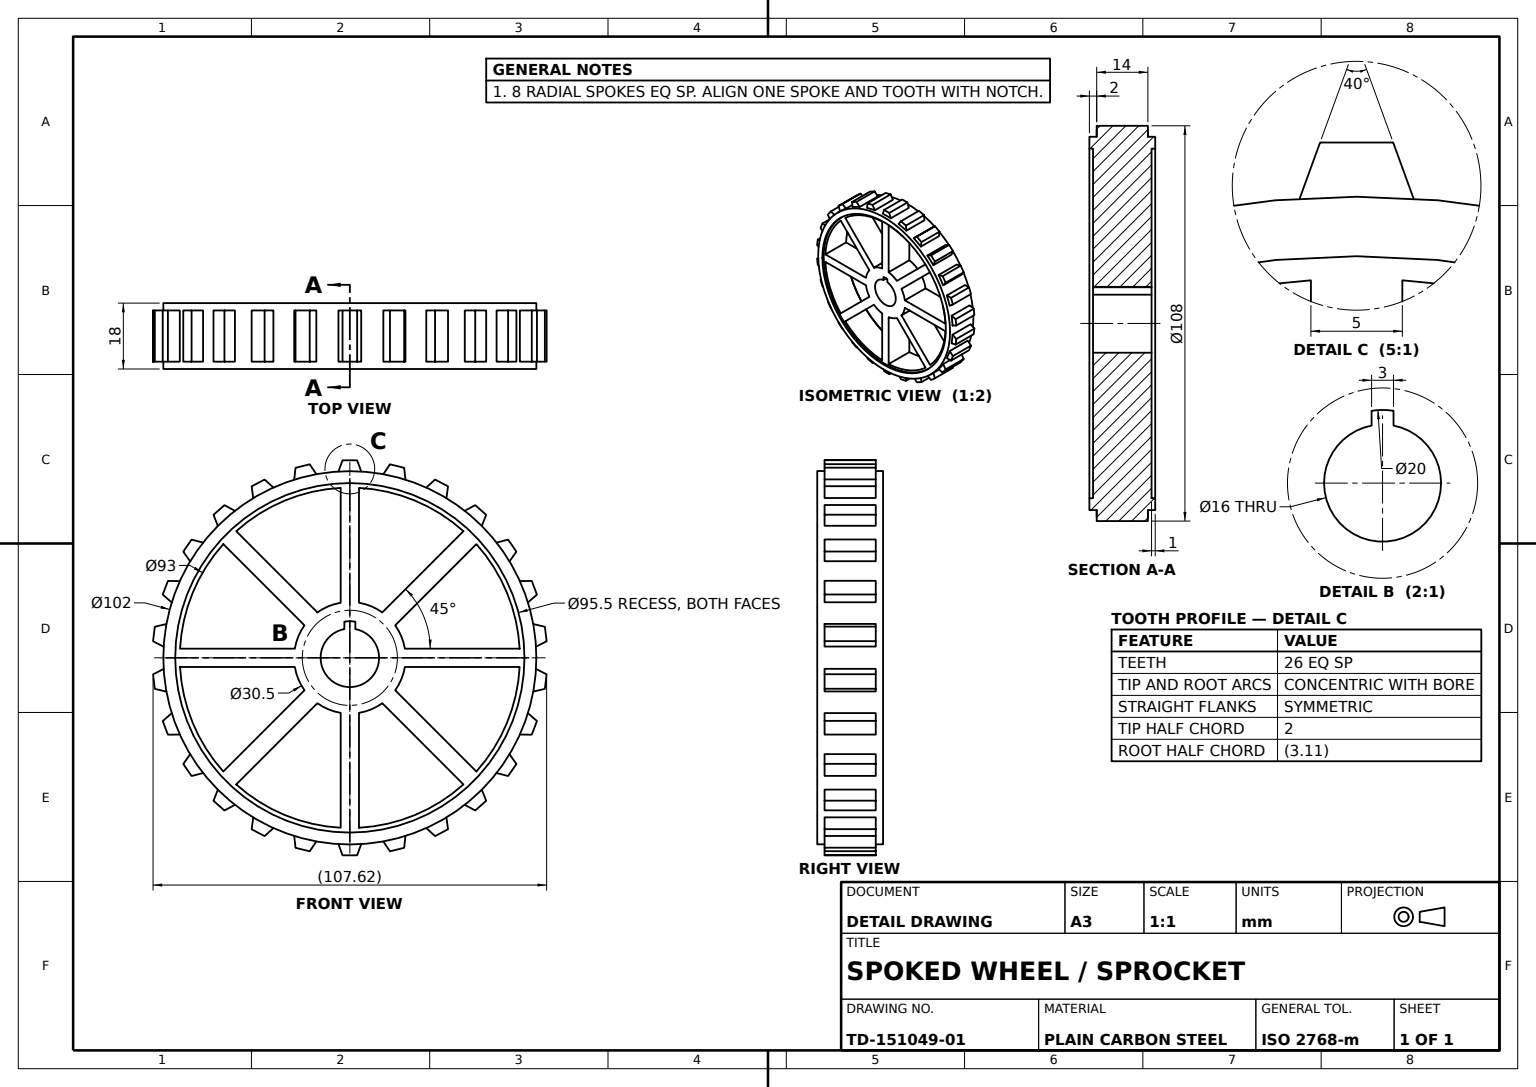
SolidWorks part; units mm, degrees
material "Plain Carbon Steel"
ref_plane "Front Plane" through (0, 0, 0) normal (0, 0, 1) x (1, 0, 0)
ref_plane "Top Plane" through (0, 0, 0) normal (0, 1, 0) x (1, 0, 0)
ref_plane "Right Plane" through (0, 0, 0) normal (1, 0, 0) x (0, 0, -1)
sketch "Hub Spokes Rim Sketch" plane through (0, 0, 0) normal (0, 0, 1) x (1, 0, 0)
  line L0 (0, 0) -> (0, 62.7961) construction
  line L1 (-2.5, 15.0437) -> (-2.5, 46.4327)
  line L2 (2.5, 46.4327) -> (2.5, 15.0437)
  line L3 (34.6007, 31.0651) -> (12.4053, 8.8697)
  line L4 (8.8697, 12.4053) -> (31.0651, 34.6007)
  line L5 (46.4327, -2.5) -> (15.0437, -2.5)
  line L6 (15.0437, 2.5) -> (46.4327, 2.5)
  line L7 (31.0651, -34.6007) -> (8.8697, -12.4053)
  line L8 (12.4053, -8.8697) -> (34.6007, -31.0651)
  line L9 (-2.5, -46.4327) -> (-2.5, -15.0437)
  line L10 (2.5, -15.0437) -> (2.5, -46.4327)
  line L11 (-34.6007, -31.0651) -> (-12.4053, -8.8697)
  line L12 (-8.8697, -12.4053) -> (-31.0651, -34.6007)
  line L13 (-46.4327, 2.5) -> (-15.0437, 2.5)
  line L14 (-15.0437, -2.5) -> (-46.4327, -2.5)
  line L15 (-31.0651, 34.6007) -> (-8.8697, 12.4053)
  line L16 (-12.4053, 8.8697) -> (-34.6007, 31.0651)
  circle A0 centre (0, 0) radius 51
  arc A1 (-2.5, 15.0437) -> (-8.8697, 12.4053) centre (0, 0) ccw
  circle A2 centre (0, 0) radius 8
  arc A3 (-2.5, 46.4327) -> (-31.0651, 34.6007) centre (0, 0) ccw
  arc A4 (8.8697, 12.4053) -> (2.5, 15.0437) centre (0, 0) ccw
  arc A5 (15.0437, 2.5) -> (12.4053, 8.8697) centre (0, 0) ccw
  arc A6 (12.4053, -8.8697) -> (15.0437, -2.5) centre (0, 0) ccw
  arc A7 (2.5, -15.0437) -> (8.8697, -12.4053) centre (0, 0) ccw
  arc A8 (-8.8697, -12.4053) -> (-2.5, -15.0437) centre (0, 0) ccw
  arc A9 (-15.0437, -2.5) -> (-12.4053, -8.8697) centre (0, 0) ccw
  arc A10 (-12.4053, 8.8697) -> (-15.0437, 2.5) centre (0, 0) ccw
  arc A11 (31.0651, 34.6007) -> (2.5, 46.4327) centre (0, 0) ccw
  arc A12 (46.4327, 2.5) -> (34.6007, 31.0651) centre (0, 0) ccw
  arc A13 (34.6007, -31.0651) -> (46.4327, -2.5) centre (0, 0) ccw
  arc A14 (2.5, -46.4327) -> (31.0651, -34.6007) centre (0, 0) ccw
  arc A15 (-31.0651, -34.6007) -> (-2.5, -46.4327) centre (0, 0) ccw
  arc A16 (-46.4327, -2.5) -> (-34.6007, -31.0651) centre (0, 0) ccw
  arc A17 (-34.6007, 31.0651) -> (-46.4327, 2.5) centre (0, 0) ccw
  point P41 (0, 0)
  dimension "D1" = 16
  dimension "D2" = 30.5
  dimension "D3" = 93
  dimension "D4" = 102
  dimension "D5" = 5
  dimension "D6" = 2.5
  dimension "D7" = 8
extrude "Wheel Body 8 Spokes" add sketch "Hub Spokes Rim Sketch" along normal mid plane 18 contours L14 A16 L11 A9
sketch "Teeth Profile Sketch 26x" plane through (0, 0, 0) normal (0, 0, 1) x (1, 0, 0)
  line L0 (10.9723, 52.8735) -> (9.1598, 50.1707)
  line L1 (-2, 53.963) -> (-3.113, 50.9049)
  line L2 (2, 53.963) -> (3.113, 50.9049)
  line L3 (14.8561, 51.9163) -> (15.2049, 48.6807)
  line L4 (23.3069, 48.7113) -> (20.9002, 46.5208)
  line L5 (26.8487, 46.8524) -> (26.4131, 43.6274)
  line L6 (34.287, 41.7181) -> (31.4261, 40.1672)
  line L7 (37.2811, 39.0656) -> (36.0863, 36.0385)
  line L8 (43.2745, 32.3004) -> (40.1255, 31.4793)
  line L9 (45.5468, 29.0085) -> (43.6623, 26.3553)
  line L10 (49.747, 21.0056) -> (46.493, 20.9619)
  line L11 (51.1654, 17.2655) -> (48.7008, 15.1404)
  line L12 (53.3284, 8.4899) -> (50.1585, 9.2262)
  line L13 (53.8106, 4.5191) -> (50.909, 3.0456)
  line L14 (53.8106, -4.5191) -> (50.909, -3.0456)
  line L15 (53.3284, -8.4899) -> (50.1585, -9.2262)
  line L16 (51.1654, -17.2655) -> (48.7008, -15.1404)
  line L17 (49.747, -21.0056) -> (46.493, -20.9619)
  line L18 (45.5468, -29.0085) -> (43.6623, -26.3553)
  line L19 (43.2745, -32.3004) -> (40.1255, -31.4793)
  line L20 (37.2811, -39.0656) -> (36.0863, -36.0385)
  line L21 (34.287, -41.7181) -> (31.4261, -40.1672)
  line L22 (26.8487, -46.8524) -> (26.4131, -43.6274)
  line L23 (23.3069, -48.7113) -> (20.9002, -46.5208)
  line L24 (14.8561, -51.9163) -> (15.2049, -48.6807)
  line L25 (10.9723, -52.8735) -> (9.1598, -50.1707)
  line L26 (2, -53.963) -> (3.113, -50.9049)
  line L27 (-2, -53.963) -> (-3.113, -50.9049)
  line L28 (-10.9723, -52.8735) -> (-9.1598, -50.1707)
  line L29 (-14.8561, -51.9163) -> (-15.2049, -48.6807)
  line L30 (-23.3069, -48.7113) -> (-20.9002, -46.5208)
  line L31 (-26.8487, -46.8524) -> (-26.4131, -43.6274)
  line L32 (-34.287, -41.7181) -> (-31.4261, -40.1672)
  line L33 (-37.2811, -39.0656) -> (-36.0863, -36.0385)
  line L34 (-43.2745, -32.3004) -> (-40.1255, -31.4793)
  line L35 (-45.5468, -29.0085) -> (-43.6623, -26.3553)
  line L36 (-49.747, -21.0056) -> (-46.493, -20.9619)
  line L37 (-51.1654, -17.2655) -> (-48.7008, -15.1404)
  line L38 (-53.3284, -8.4899) -> (-50.1585, -9.2262)
  line L39 (-53.8106, -4.5191) -> (-50.909, -3.0456)
  line L40 (-53.8106, 4.5191) -> (-50.909, 3.0456)
  line L41 (-53.3284, 8.4899) -> (-50.1585, 9.2262)
  line L42 (-51.1654, 17.2655) -> (-48.7008, 15.1404)
  line L43 (-49.747, 21.0056) -> (-46.493, 20.9619)
  line L44 (-45.5468, 29.0085) -> (-43.6623, 26.3553)
  line L45 (-43.2745, 32.3004) -> (-40.1255, 31.4793)
  line L46 (-37.2811, 39.0656) -> (-36.0863, 36.0385)
  line L47 (-34.287, 41.7181) -> (-31.4261, 40.1672)
  line L48 (-26.8487, 46.8524) -> (-26.4131, 43.6274)
  line L49 (-23.3069, 48.7113) -> (-20.9002, 46.5208)
  line L50 (-14.8561, 51.9163) -> (-15.2049, 48.6807)
  line L51 (-10.9723, 52.8735) -> (-9.1598, 50.1707)
  arc A0 (2, 53.963) -> (-2, 53.963) centre (0, 0) ccw
  circle A1 centre (0, 0) radius 51 construction
  arc A2 (-3.113, 50.9049) -> (-9.1598, 50.1707) centre (0, 0) ccw
  arc A3 (14.8561, 51.9163) -> (10.9723, 52.8735) centre (0, 0) ccw
  arc A4 (26.8487, 46.8524) -> (23.3069, 48.7113) centre (0, 0) ccw
  arc A5 (37.2811, 39.0656) -> (34.287, 41.7181) centre (0, 0) ccw
  arc A6 (45.5468, 29.0085) -> (43.2745, 32.3004) centre (0, 0) ccw
  arc A7 (51.1654, 17.2655) -> (49.747, 21.0056) centre (0, 0) ccw
  arc A8 (53.8106, 4.5191) -> (53.3284, 8.4899) centre (0, 0) ccw
  arc A9 (53.3284, -8.4899) -> (53.8106, -4.5191) centre (0, 0) ccw
  arc A10 (49.747, -21.0056) -> (51.1654, -17.2655) centre (0, 0) ccw
  arc A11 (43.2745, -32.3004) -> (45.5468, -29.0085) centre (0, 0) ccw
  arc A12 (34.287, -41.7181) -> (37.2811, -39.0656) centre (0, 0) ccw
  arc A13 (23.3069, -48.7113) -> (26.8487, -46.8524) centre (0, 0) ccw
  arc A14 (10.9723, -52.8735) -> (14.8561, -51.9163) centre (0, 0) ccw
  arc A15 (-2, -53.963) -> (2, -53.963) centre (0, 0) ccw
  arc A16 (-14.8561, -51.9163) -> (-10.9723, -52.8735) centre (0, 0) ccw
  arc A17 (-26.8487, -46.8524) -> (-23.3069, -48.7113) centre (0, 0) ccw
  arc A18 (-37.2811, -39.0656) -> (-34.287, -41.7181) centre (0, 0) ccw
  arc A19 (-45.5468, -29.0085) -> (-43.2745, -32.3004) centre (0, 0) ccw
  arc A20 (-51.1654, -17.2655) -> (-49.747, -21.0056) centre (0, 0) ccw
  arc A21 (-53.8106, -4.5191) -> (-53.3284, -8.4899) centre (0, 0) ccw
  arc A22 (-53.3284, 8.4899) -> (-53.8106, 4.5191) centre (0, 0) ccw
  arc A23 (-49.747, 21.0056) -> (-51.1654, 17.2655) centre (0, 0) ccw
  arc A24 (-43.2745, 32.3004) -> (-45.5468, 29.0085) centre (0, 0) ccw
  arc A25 (-34.287, 41.7181) -> (-37.2811, 39.0656) centre (0, 0) ccw
  arc A26 (-23.3069, 48.7113) -> (-26.8487, 46.8524) centre (0, 0) ccw
  arc A27 (-10.9723, 52.8735) -> (-14.8561, 51.9163) centre (0, 0) ccw
  arc A28 (-15.2049, 48.6807) -> (-20.9002, 46.5208) centre (0, 0) ccw
  arc A29 (-26.4131, 43.6274) -> (-31.4261, 40.1672) centre (0, 0) ccw
  arc A30 (-36.0863, 36.0385) -> (-40.1255, 31.4793) centre (0, 0) ccw
  arc A31 (-43.6623, 26.3553) -> (-46.493, 20.9619) centre (0, 0) ccw
  arc A32 (-48.7008, 15.1404) -> (-50.1585, 9.2262) centre (0, 0) ccw
  arc A33 (-50.909, 3.0456) -> (-50.909, -3.0456) centre (0, 0) ccw
  arc A34 (-50.1585, -9.2262) -> (-48.7008, -15.1404) centre (0, 0) ccw
  arc A35 (-46.493, -20.9619) -> (-43.6623, -26.3553) centre (0, 0) ccw
  arc A36 (-40.1255, -31.4793) -> (-36.0863, -36.0385) centre (0, 0) ccw
  arc A37 (-31.4261, -40.1672) -> (-26.4131, -43.6274) centre (0, 0) ccw
  arc A38 (-20.9002, -46.5208) -> (-15.2049, -48.6807) centre (0, 0) ccw
  arc A39 (-9.1598, -50.1707) -> (-3.113, -50.9049) centre (0, 0) ccw
  arc A40 (3.113, -50.9049) -> (9.1598, -50.1707) centre (0, 0) ccw
  arc A41 (15.2049, -48.6807) -> (20.9002, -46.5208) centre (0, 0) ccw
  arc A42 (26.4131, -43.6274) -> (31.4261, -40.1672) centre (0, 0) ccw
  arc A43 (36.0863, -36.0385) -> (40.1255, -31.4793) centre (0, 0) ccw
  arc A44 (43.6623, -26.3553) -> (46.493, -20.9619) centre (0, 0) ccw
  arc A45 (48.7008, -15.1404) -> (50.1585, -9.2262) centre (0, 0) ccw
  arc A46 (50.909, -3.0456) -> (50.909, 3.0456) centre (0, 0) ccw
  arc A47 (50.1585, 9.2262) -> (48.7008, 15.1404) centre (0, 0) ccw
  arc A48 (46.493, 20.9619) -> (43.6623, 26.3553) centre (0, 0) ccw
  arc A49 (40.1255, 31.4793) -> (36.0863, 36.0385) centre (0, 0) ccw
  arc A50 (31.4261, 40.1672) -> (26.4131, 43.6274) centre (0, 0) ccw
  arc A51 (20.9002, 46.5208) -> (15.2049, 48.6807) centre (0, 0) ccw
  arc A52 (9.1598, 50.1707) -> (3.113, 50.9049) centre (0, 0) ccw
  point P111 (0, 0)
  dimension "D1" = 108
  dimension "D2" = 2
  dimension "D3" = 3.113
  dimension "D4" = 26
extrude "Teeth Ring 26x" add sketch "Teeth Profile Sketch 26x" along normal mid plane 14
sketch "Web Pockets Sketch 8x" plane through (0, 0, 7) normal (0, 0, 1) x (1, 0, 0)
  line L0 (2.5, 15.0437) -> (2.5, 46.4327)
  line L1 (2.5, 46.4327) -> (2.5, 15.0437) construction
  line L2 (8.8697, 12.4053) -> (31.0651, 34.6007)
  line L3 (12.4053, 8.8697) -> (34.6007, 31.0651)
  line L4 (15.0437, 2.5) -> (46.4327, 2.5)
  line L5 (15.0437, -2.5) -> (46.4327, -2.5)
  line L6 (12.4053, -8.8697) -> (34.6007, -31.0651)
  line L7 (8.8697, -12.4053) -> (31.0651, -34.6007)
  line L8 (2.5, -15.0437) -> (2.5, -46.4327)
  line L9 (-2.5, -15.0437) -> (-2.5, -46.4327)
  line L10 (-8.8697, -12.4053) -> (-31.0651, -34.6007)
  line L11 (-12.4053, -8.8697) -> (-34.6007, -31.0651)
  line L12 (-15.0437, -2.5) -> (-46.4327, -2.5)
  line L13 (-15.0437, 2.5) -> (-46.4327, 2.5)
  line L14 (-12.4053, 8.8697) -> (-34.6007, 31.0651)
  line L15 (-8.8697, 12.4053) -> (-31.0651, 34.6007)
  line L16 (-2.5, 15.0437) -> (-2.5, 46.4327)
  arc A0 (8.8697, 12.4053) -> (2.5, 15.0437) centre (0, 0) ccw
  arc A1 (31.0651, 34.6007) -> (2.5, 46.4327) centre (0, 0) ccw
  arc A2 (15.0437, 2.5) -> (12.4053, 8.8697) centre (0, 0) ccw
  arc A3 (46.4327, 2.5) -> (34.6007, 31.0651) centre (0, 0) ccw
  arc A4 (12.4053, -8.8697) -> (15.0437, -2.5) centre (0, 0) ccw
  arc A5 (34.6007, -31.0651) -> (46.4327, -2.5) centre (0, 0) ccw
  arc A6 (2.5, -15.0437) -> (8.8697, -12.4053) centre (0, 0) ccw
  arc A7 (2.5, -46.4327) -> (31.0651, -34.6007) centre (0, 0) ccw
  arc A8 (-8.8697, -12.4053) -> (-2.5, -15.0437) centre (0, 0) ccw
  arc A9 (-31.0651, -34.6007) -> (-2.5, -46.4327) centre (0, 0) ccw
  arc A10 (-15.0437, -2.5) -> (-12.4053, -8.8697) centre (0, 0) ccw
  arc A11 (-46.4327, -2.5) -> (-34.6007, -31.0651) centre (0, 0) ccw
  arc A12 (-12.4053, 8.8697) -> (-15.0437, 2.5) centre (0, 0) ccw
  arc A13 (-34.6007, 31.0651) -> (-46.4327, 2.5) centre (0, 0) ccw
  arc A14 (-2.5, 15.0437) -> (-8.8697, 12.4053) centre (0, 0) ccw
  arc A15 (-2.5, 46.4327) -> (-31.0651, 34.6007) centre (0, 0) ccw
  point P41 (0, 0)
  dimension "D1" = 8
extrude "Web Pockets 8x" cut sketch "Web Pockets Sketch 8x" against normal through all
sketch "Hub Cut Sketch 20x16" plane through (0, 0, 9) normal (0, 0, 1) x (1, 0, 0)
  line L0 (-2.5, 15.0437) -> (-2.5, 46.4327) construction
  line L2 (1.5, 9.8869) -> (1.5, 7.8581)
  line L3 (-1.5, 9.8869) -> (-1.5, 7.8581)
  arc A0 (1.5, 9.8869) -> (-1.5, 9.8869) centre (0, 0) ccw
  arc A1 (-1.5, 7.8581) -> (1.5, 7.8581) centre (0, 0) ccw
  dimension "D1" = 20
  dimension "D2" = 16
  dimension "D3" = 1
extrude "Hub Cut 20x16" cut sketch "Hub Cut Sketch 20x16" against normal through all
sketch "Front Recess Sketch Ø95.5" plane through (0, 0, 9) normal (0, 0, 1) x (1, 0, 0)
  circle A0 centre (0, 0) radius 47.75
  dimension "D1" = 95.5
extrude "Front Face Recess Ø95.5" cut sketch "Front Recess Sketch Ø95.5" against normal blind 1
sketch "Back Recess Sketch Ø95.5" plane through (0, 0, -9) normal (0, 0, -1) x (-1, 0, 0)
  circle A0 centre (0, 0) radius 47.75
  dimension "D1" = 95.5
extrude "Back Face Recess Ø95.5" cut sketch "Back Recess Sketch Ø95.5" against normal blind 1
